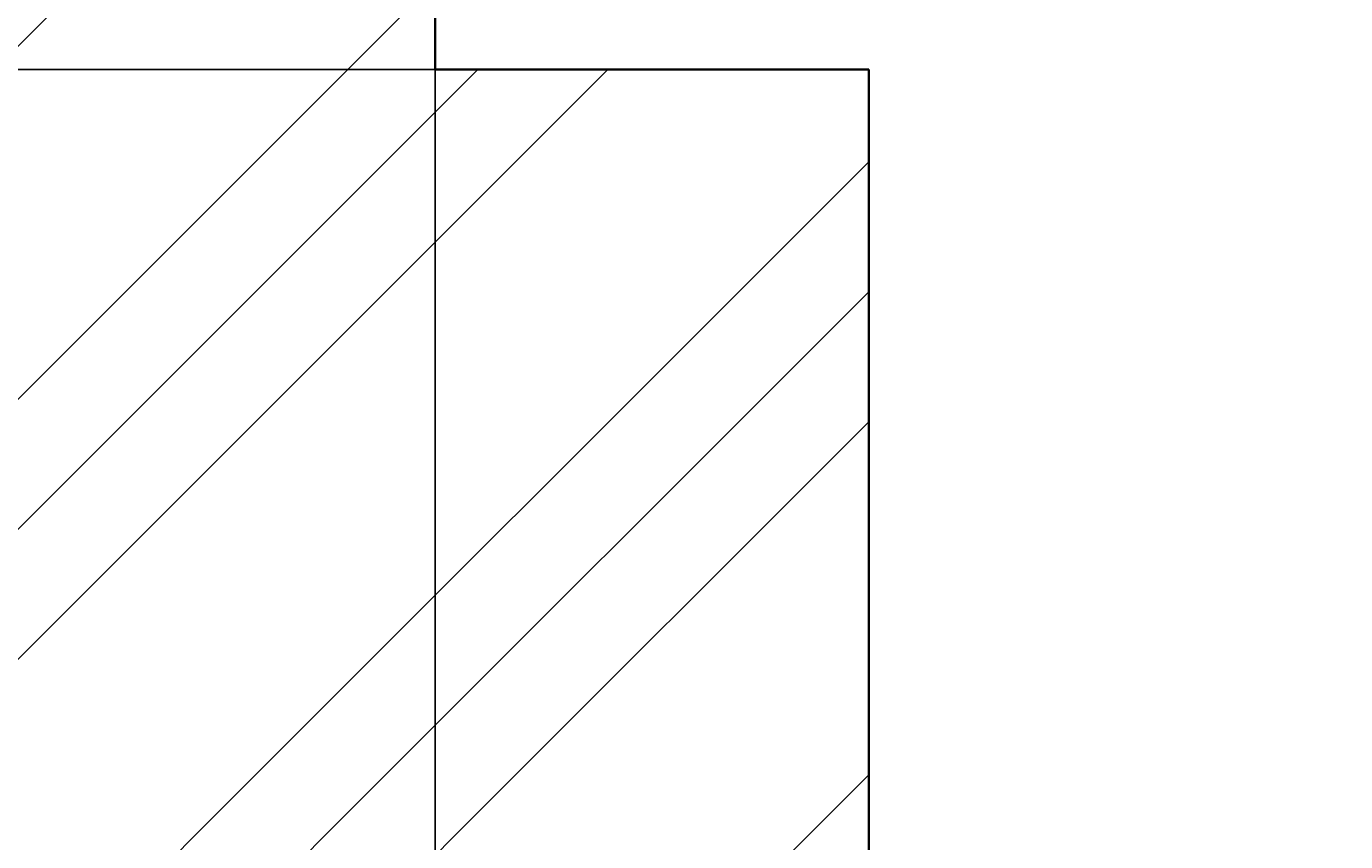
# Model space of a CAD drawing. Units: inches. Extents: x -128 to 854, y -395 to 398.
# Tile 7 of 61: x -47 to -16, y -340 to -321. Entities that reach past the tile are written whole.
import ezdxf

# ---------------------------------------------------------------- set-up
doc = ezdxf.new("R2010")
doc.units = ezdxf.units.IN
doc.header["$MEASUREMENT"] = 0
for name, color, linetype, lineweight in [('A-ANNO-DIMS', 2, 'Continuous', 18), ('A-SECT-PATT', 8, 'Continuous', 13), ('S-FNDN', 2, 'Continuous', 35)]:
    doc.layers.add(name, color=color, linetype=linetype, lineweight=lineweight)
doc.styles.get("Standard").update_dxf_attribs({"font": 'arial.ttf'})
doc.dimstyles.get("Standard").update_dxf_attribs({"dimtxt": 0.18, "dimasz": 0.18, "dimexe": 0.18, "dimexo": 0.0625, "dimgap": 0.09, "dimtad": 0, "dimtih": 1, "dimtoh": 1, "dimdec": 1, "dimzin": 0, "dimdsep": 46, "dimlunit": 4, "dimtxsty": 'Standard', "dimcen": 0.09, "dimclrd": 1, "dimclre": 2, "dimclrt": 6, "dimadec": 0, "dimazin": 0, "dimtfac": 1, "dimtdec": 1, "dimtofl": 0, "dimtmove": 0, "dimatfit": 3, "dimfxl": 1, "dimtfill": 2, "dimtfillclr": 3, "dimtolj": 1, "dimtzin": 0, "dimarcsym": 0})

# ---------------------------------------------------------------- blocks, each defined once
blk = doc.blocks.new('*D125')
at = {"layer": 'A-ANNO-DIMS', "color": 2, "lineweight": -2, "transparency": 16777216}
for p, q in [((-37.161, -298.082), (-37.161, -381.899)), ((22.811, -298.082), (22.811, -381.899))]:
    blk.add_line(p, q, dxfattribs=at)
at = {"layer": 'A-ANNO-DIMS', "color": 1, "lineweight": -2, "transparency": 16777216}
for p, q in [((-36.981, -381.719), (-7.504, -381.719)), ((22.631, -381.719), (-6.846, -381.719))]:
    blk.add_line(p, q, dxfattribs=at)
at = {"layer": 'A-ANNO-DIMS', "color": 1, "transparency": 16777216}
for points in [[(-36.981, -381.689), (-36.981, -381.749), (-37.161, -381.719)], [(22.631, -381.689), (22.631, -381.749), (22.811, -381.719)]]:
    blk.add_solid(points, dxfattribs=at)
at = {"layer": 'Defpoints', "color": 0, "transparency": 16777216}
for p in [(-37.161, -298.019), (22.811, -298.019), (22.811, -381.719)]:
    blk.add_point(p, dxfattribs=at)
at = {"layer": 'A-ANNO-DIMS', "color": 6, "transparency": 16777216, "insert": (-7.175, -381.719), "char_height": 0.18, "attachment_point": 5, "bg_fill": 1, "box_fill_scale": 1.25, "bg_fill_color": 3, "bg_fill_transparency": 0}
blk.add_mtext('\\A1;5\'-0"', dxfattribs=at)
blk = doc.blocks.new('*D129')
at = {"layer": 'A-ANNO-DIMS', "color": 2, "lineweight": -2, "transparency": 16777216}
for p, q in [((-27.223, -322.019), (-128.041, -322.019)), ((-27.223, -346.019), (-128.041, -346.019))]:
    blk.add_line(p, q, dxfattribs=at)
at = {"layer": 'A-ANNO-DIMS', "color": 1, "lineweight": -2, "transparency": 16777216}
for p, q in [((-127.861, -322.199), (-127.861, -333.837)), ((-127.861, -345.839), (-127.861, -334.201))]:
    blk.add_line(p, q, dxfattribs=at)
at = {"layer": 'A-ANNO-DIMS', "color": 1, "transparency": 16777216}
for points in [[(-127.891, -322.199), (-127.831, -322.199), (-127.861, -322.019)], [(-127.891, -345.839), (-127.831, -345.839), (-127.861, -346.019)]]:
    blk.add_solid(points, dxfattribs=at)
at = {"layer": 'Defpoints', "color": 0, "transparency": 16777216}
for p in [(-127.861, -322.019), (-27.161, -322.019), (-27.161, -346.019)]:
    blk.add_point(p, dxfattribs=at)
at = {"layer": 'A-ANNO-DIMS', "color": 6, "transparency": 16777216, "insert": (-127.861, -334.019), "char_height": 0.18, "attachment_point": 5, "bg_fill": 1, "box_fill_scale": 1.25, "bg_fill_color": 3, "bg_fill_transparency": 0}
blk.add_mtext('\\A1;2\'-0"', dxfattribs=at)
blk = doc.blocks.new('*D130')
at = {"layer": 'A-ANNO-DIMS', "color": 2, "lineweight": -2, "transparency": 16777216}
for p, q in [((-66.161, -322.082), (-66.161, -381.899)), ((-27.161, -322.082), (-27.161, -381.899))]:
    blk.add_line(p, q, dxfattribs=at)
at = {"layer": 'A-ANNO-DIMS', "color": 1, "lineweight": -2, "transparency": 16777216}
for p, q in [((-65.981, -381.719), (-46.99, -381.719)), ((-27.341, -381.719), (-46.332, -381.719))]:
    blk.add_line(p, q, dxfattribs=at)
at = {"layer": 'A-ANNO-DIMS', "color": 1, "transparency": 16777216}
for points in [[(-65.981, -381.689), (-65.981, -381.749), (-66.161, -381.719)], [(-27.341, -381.689), (-27.341, -381.749), (-27.161, -381.719)]]:
    blk.add_solid(points, dxfattribs=at)
at = {"layer": 'Defpoints', "color": 0, "transparency": 16777216}
for p in [(-66.161, -322.019), (-27.161, -322.019), (-27.161, -381.719)]:
    blk.add_point(p, dxfattribs=at)
at = {"layer": 'A-ANNO-DIMS', "color": 6, "transparency": 16777216, "insert": (-46.661, -381.719), "char_height": 0.18, "attachment_point": 5, "bg_fill": 1, "box_fill_scale": 1.25, "bg_fill_color": 3, "bg_fill_transparency": 0}
blk.add_mtext('\\A1;3\'-3"', dxfattribs=at)

msp = doc.modelspace()

# ---------------------------------------------------------------- hatches: boundary and pattern name
at = {"layer": 'A-SECT-PATT'}
h = msp.add_hatch(dxfattribs=at)
h.set_pattern_fill('GOST_GROUND', color=256)
h.set_pattern_definition([(45, (0, 0), (14.14214, -9e-16), [20]), (45, (3, 0), (14.14214, -9e-16), [20]), (45, (6, 0), (14.14214, -9e-16), [20])])
h.paths.add_polyline_path([(-27.161, -322.019), (-37.161, -322.019), (-37.161, -298.019), (-56.161, -298.019), (-56.161, -322.019), (-66.161, -322.019), (-66.161, -346.019), (-27.161, -346.019)])
h.paths.add_polyline_path([(170.839, -322.019), (160.839, -322.019), (160.839, -298.019), (155.839, -298.019), (141.839, -298.019), (141.839, -322.019), (131.839, -322.019), (131.839, -346.019), (170.839, -346.019)])
h.paths.add_polyline_path([(327.839, -322.019), (317.839, -322.019), (317.839, -298.019), (312.839, -298.019), (298.839, -298.019), (298.839, -322.019), (288.839, -322.019), (288.839, -346.019), (327.839, -346.019)])
h.paths.add_polyline_path([(-37.161, -274.019), (-56.161, -274.019), (-56.161, -298.019), (-37.161, -298.019)])
h.paths.add_polyline_path([(-37.161, -207.019), (-56.161, -207.019), (-56.161, -226.019), (-37.161, -226.019)])
h.paths.add_polyline_path([(160.839, -274.019), (141.839, -274.019), (141.839, -298.019), (155.839, -298.019), (160.839, -298.019)])

# ---------------------------------------------------------------- linework, layer by layer
at = {"layer": 'S-FNDN'}
for p, q in [((-37.161, -298.019), (-37.161, -322.019)), ((-37.161, -322.019), (-27.161, -322.019)), ((-27.161, -322.019), (-27.161, -346.019))]:
    msp.add_line(p, q, dxfattribs=at)

# ---------------------------------------------------------------- dimensions: what is measured, and where the dimension line sits
at = {"layer": 'A-ANNO-DIMS'}
for base, p1, p2, picture, middle in [((22.811, -381.719), (-37.161, -298.019), (22.811, -298.019), '*D125', (-7.175, -381.719)), ((-27.161, -381.719), (-66.161, -322.019), (-27.161, -322.019), '*D130', (-46.661, -381.719))]:
    dim = msp.add_linear_dim(base=base, p1=p1, p2=p2, dimstyle='Standard', override={"dimdec": 1, "dimlfac": 1, "dimrnd": 0, "dimzin": 1, "dimdsep": 46, "dimlunit": 4, "dimfrac": 2}, dxfattribs=at)
    dim.commit()
    dim.dimension.update_dxf_attribs({"geometry": picture, "text_midpoint": middle})
dim = msp.add_linear_dim(base=(-127.861, -322.019), p1=(-27.161, -346.019), p2=(-27.161, -322.019), angle=90, dimstyle='Standard', override={"dimdec": 1, "dimlfac": 1, "dimrnd": 0, "dimzin": 1, "dimdsep": 46, "dimlunit": 4, "dimfrac": 2}, dxfattribs=at)
dim.commit()
dim.dimension.update_dxf_attribs({"geometry": '*D129', "text_midpoint": (-127.861, -334.019)})

doc.saveas('drawing.dxf')
